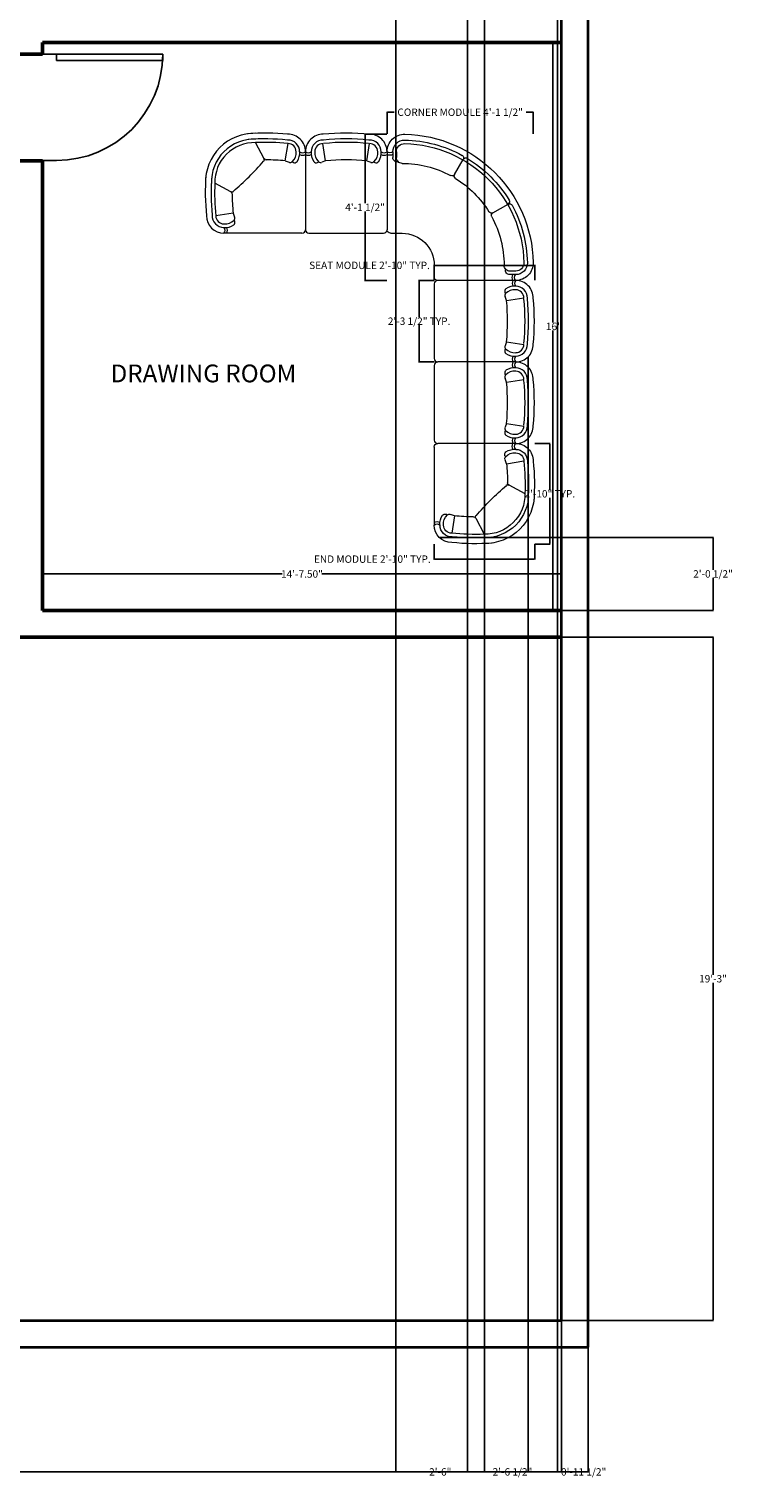
# Model space of a CAD drawing. Units: inches. Extents: x 594 to 1173, y 353 to 1285.
# Tile 3 of 6: x 934 to 1172, y 353 to 844. Entities that reach past the tile are written whole.
import ezdxf

# ---------------------------------------------------------------- set-up
doc = ezdxf.new("R2010")
doc.units = ezdxf.units.IN
doc.header["$MEASUREMENT"] = 0
for name, color, linetype, lineweight in [('A-ANNO-DIMS', 2, 'Continuous', 18), ('A-AREA-IDEN', 7, 'Continuous', 25), ('A-DOOR', 4, 'Continuous', 25), ('A-FURN', 8, 'Continuous', 18), ('A-WALL', 7, 'Continuous', 50), ('C-PROP', 7, 'Continuous', 35)]:
    doc.layers.add(name, color=color, linetype=linetype, lineweight=lineweight)
doc.styles.get("Standard").update_dxf_attribs({"font": 'arial.ttf'})
doc.dimstyles.get("Standard").update_dxf_attribs({"dimtxt": 2.5, "dimasz": 0.18, "dimexe": 0.18, "dimexo": 0.0625, "dimgap": 0.09, "dimtad": 0, "dimtih": 1, "dimtoh": 1, "dimzin": 0, "dimdsep": 46, "dimlunit": 3, "dimtxsty": 'Standard', "dimcen": 0.09, "dimadec": 0, "dimazin": 0, "dimtfac": 1, "dimtofl": 0, "dimtmove": 0, "dimatfit": 3, "dimfxl": 1, "dimtolj": 1, "dimtzin": 0, "dimarcsym": 0})

# ---------------------------------------------------------------- blocks, each defined once
blk = doc.blocks.new('*U2')
for p, q in [((0, 0), (0, -100)), ((750, 0), (750, -100))]:
    blk.add_line(p, q)
blk.add_lwpolyline([(0, 0), (0, 750), (43.75, 750), (43.75, 0)], close=True)
blk.add_arc((0, 0), 750, 0, 90)
blk = doc.blocks.new('A$C707258B2')
at = {"color": 0}
for p, q in [((0.404, 0.342), (1.074, 0.342)), ((0.404, 0.292), (0.454, 0.292)), ((0.404, 0.262), (0.454, 0.262)), ((1.104, 0.312), (1.104, 0.212)), ((1.479, -0.063), (1.379, -0.063)), ((1.509, -0.763), (1.509, -0.093)), ((0.6, -0.238), (0.47, -0.313)), ((0.929, -0.567), (0.854, -0.697)), ((1.429, -0.763), (1.429, -0.713)), ((1.459, -0.763), (1.459, -0.712))]:
    blk.add_line(p, q, dxfattribs=at)
for centre, radius, start, end in [((0.404, 0.192), 0.15, 90, 181.1754), ((0.404, 0.192), 0.1, 90, 181.1754), ((0.404, 0.192), 0.07, 90, 181.1754), ((0.378, 0.317), 0.0362, 316.3972, 43.6028), ((0.368, 0.317), 0.0662, 337.8298, 22.1702), ((0.455, 0.256), 0.0357, 345.4262, 90.5555), ((0.454, 0.212), 0.05, 360, 90), ((1.074, 0.312), 0.03, 360, 90), ((1.379, 0.212), 1.125, 181.1754, 268.8246), ((1.379, 0.212), 1.075, 181.1754, 208.6357), ((1.379, 0.212), 1.045, 181.1754, 268.8246), ((1.379, 0.212), 0.875, 180, 208.4082), ((1.379, 0.212), 0.275, 180, 270), ((1.479, -0.093), 0.03, 360, 90), ((0.587, -0.216), 0.025, 300, 28.4082), ((0.612, -0.259), 0.025, 31.5918, 120), ((1.379, 0.212), 0.875, 211.5918, 238.4082), ((0.457, -0.291), 0.025, 208.6357, 300), ((0.482, -0.334), 0.025, 120, 211.3643), ((1.379, 0.212), 1.075, 211.3643, 238.6357), ((0.907, -0.555), 0.025, 330, 58.4082), ((0.951, -0.58), 0.025, 61.5918, 150), ((1.379, 0.212), 0.875, 241.5918, 270), ((0.832, -0.685), 0.025, 238.6357, 330), ((0.876, -0.71), 0.025, 150, 241.3643), ((1.379, 0.212), 1.075, 241.3643, 268.8246), ((1.379, -0.713), 0.05, 360, 90), ((1.425, -0.709), 0.0336, 354.6301, 109.3883), ((1.484, -0.799), 0.0662, 67.8298, 112.1702), ((1.359, -0.763), 0.15, 268.8246, 360), ((1.359, -0.763), 0.1, 268.8246, 360), ((1.359, -0.763), 0.07, 268.8246, 360), ((1.484, -0.789), 0.0362, 46.3972, 133.6028)]:
    blk.add_arc(centre, radius, start, end, dxfattribs=at)
blk = doc.blocks.new('part 01')
at = {"color": 0}
for p, q in [((-670, 700), (0, 700)), ((30, 30), (30, 670)), ((-591, 527), (-740, 550)), ((-591, 527), (-579, 561)), ((-591, 173), (-740, 150)), ((-591, 173), (-579, 139)), ((-670, 0), (0, 0))]:
    blk.add_line(p, q, dxfattribs=at)
for centre, radius, start, end in [((-670, 550), 150, 90, 181.1754), ((-670, 550), 100, 90, 181.1754), ((-660, 518), 133, 56.0897, 95.6132), ((-696, 675), 36.2, 316.3972, 43.6028), ((-706, 675), 66.2, 337.8298, 22.1702), ((-600, 607), 25, 332.9608, 56.0897), ((0, 670), 30, 0, 90), ((1178, 350), 2008, 174.2835, 185.7165), ((1178, 350), 1958, 174.2835, 185.7165), ((1178, 350), 1928, 174.2835, 185.7165), ((-670, 550), 70, 90, 181.1754), ((-660, 518), 103, 42.0066, 95.6132), ((1178, 350), 1778, 174.2835, 185.7165), ((-625, 620), 53.2, 321.0017, 332.9608), ((-602, 570), 25, 340, 42.0066), ((-670, 150), 150, 178.8246, 270), ((-670, 150), 100, 178.8246, 270), ((-670, 150), 70, 178.8246, 270), ((-602, 130), 25, 317.9934, 20), ((-660, 182), 133, 264.3868, 303.9103), ((-660, 182), 103, 264.3868, 317.9934), ((-696, 25), 36.2, 316.3972, 43.6028), ((-706, 25), 66.2, 337.8298, 22.1702), ((-600, 93), 25, 303.9103, 27.0392), ((-625, 80), 53.2, 27.0392, 38.9983), ((0, 30), 30, 270, 0)]:
    blk.add_arc(centre, radius, start, end, dxfattribs=at)
blk = doc.blocks.new('part02')
at = {"color": 0}
for p, q in [((0, -670), (0, 0)), ((30, 30), (700, 30)), ((621, -143), (609, -109)), ((621, -143), (770, -120)), ((640, -326), (778, -399)), ((173, -591), (139, -579)), ((173, -591), (150, -740)), ((356, -610), (429, -748))]:
    blk.add_line(p, q, dxfattribs=at)
for centre, radius, start, end in [((30, 0), 30, 90, 180), ((726, 5), 56.2, 153.6122, 206.6666), ((726, 5), 36.2, 136.3972, 223.6028), ((700, -120), 150, 0, 90), ((630, -63), 25, 123.9103, 207.0392), ((655, -50), 53.2, 207.0392, 218.9983), ((632, -100), 25, 137.9934, 200), ((690, -152), 103, 84.3868, 137.9934), ((689, -151), 132, 85.4378, 123.9887), ((700, -121), 101, 357.5006, 89.858), ((700, -120), 70, 0, 90), ((-1228, -320), 2008, 357.7349, 5.7032), ((-1148, -320), 2008, 355.818, 5.7165), ((-1148, -320), 1778, 0.3836, 5.7165), ((-1148, -320), 1958, 355.8657, 5.7165), ((2220, -2190), 2454, 130.6961, 139.3039), ((632, -344), 20, 62, 130.6961), ((650, -308), 20, 180.3836, 242), ((439, -409), 419, 268.2181, 1.7819), ((439, -409), 369, 268.2181, 1.7819), ((439, -409), 339, 268.2181, 1.7819), ((182, -660), 133, 146.0897, 185.6132), ((93, -600), 25, 62.9608, 146.0897), ((182, -660), 103, 132.0066, 185.6132), ((80, -625), 53.2, 51.0017, 62.9608), ((130, -602), 25, 70, 132.0066), ((350, 1178), 1778, 264.2835, 269.6164), ((338, -620), 20, 28, 89.6164), ((374, -602), 20, 139.3039, 208), ((25, -696), 56.2, 63.3334, 116.3878), ((25, -696), 36.2, 46.3972, 133.6028), ((150, -670), 150, 180, 271.1754), ((150, -670), 100, 180, 271.1754), ((150, -670), 70, 180, 270), ((350, 1258), 2008, 264.2968, 272.2651), ((350, 1178), 2008, 264.2835, 274.182), ((350, 1178), 1958, 264.2835, 274.1343)]:
    blk.add_arc(centre, radius, start, end, dxfattribs=at)
blk = doc.blocks.new('*D19')
at = {"layer": 'A-ANNO-DIMS', "color": 0, "lineweight": -2, "transparency": 16777216}
for p, q in [((1114.27, 839.78), (1111.25, 839.78)), ((1111.43, 839.6), (1111.43, 745.15)), ((1111.43, 647.96), (1111.43, 742.42)), ((1114.27, 647.78), (1111.25, 647.78))]:
    blk.add_line(p, q, dxfattribs=at)
at = {"layer": 'A-ANNO-DIMS', "color": 0, "transparency": 16777216}
for points in [[(1111.4, 839.6), (1111.46, 839.6), (1111.43, 839.78)], [(1111.4, 647.96), (1111.46, 647.96), (1111.43, 647.78)]]:
    blk.add_solid(points, dxfattribs=at)
at = {"layer": 'Defpoints', "color": 0, "transparency": 16777216}
for p in [(1114.34, 839.78), (1111.43, 647.78), (1114.34, 647.78)]:
    blk.add_point(p, dxfattribs=at)
at = {"layer": 'A-ANNO-DIMS', "color": 0, "transparency": 16777216, "insert": (1111.43, 743.78), "char_height": 2.5, "attachment_point": 5}
blk.add_mtext("\\A1;16'", dxfattribs=at)
blk = doc.blocks.new('*D20')
at = {"layer": 'A-ANNO-DIMS', "color": 0, "lineweight": -2, "transparency": 16777216}
for p, q in [((938.84, 647.85), (938.84, 660.27)), ((939.02, 660.09), (1019.89, 660.09)), ((1114.16, 660.09), (1033.28, 660.09)), ((1114.34, 647.85), (1114.34, 660.27))]:
    blk.add_line(p, q, dxfattribs=at)
at = {"layer": 'A-ANNO-DIMS', "color": 0, "transparency": 16777216}
for points in [[(939.02, 660.12), (939.02, 660.06), (938.84, 660.09)], [(1114.16, 660.12), (1114.16, 660.06), (1114.34, 660.09)]]:
    blk.add_solid(points, dxfattribs=at)
at = {"layer": 'Defpoints', "color": 0, "transparency": 16777216}
for p in [(1114.34, 660.09), (938.84, 647.78), (1114.34, 647.78)]:
    blk.add_point(p, dxfattribs=at)
at = {"layer": 'A-ANNO-DIMS', "color": 0, "transparency": 16777216, "insert": (1026.59, 660.09), "char_height": 2.5, "attachment_point": 5}
blk.add_mtext('\\A1;14\'-7.50"', dxfattribs=at)
blk = doc.blocks.new('*D38')
at = {"layer": 'A-ANNO-DIMS', "color": 0, "lineweight": -2, "transparency": 16777216}
for p, q in [((1071.29, 764.42), (1071.11, 764.42)), ((1071.29, 759.38), (1071.29, 764.6)), ((1105.1, 764.42), (1071.47, 764.42)), ((1105.28, 759.38), (1105.28, 764.6))]:
    blk.add_line(p, q, dxfattribs=at)
at = {"layer": 'A-ANNO-DIMS', "color": 0, "transparency": 16777216}
for points in [[(1071.47, 764.45), (1071.47, 764.39), (1071.29, 764.42)], [(1105.1, 764.45), (1105.1, 764.39), (1105.28, 764.42)]]:
    blk.add_solid(points, dxfattribs=at)
at = {"layer": 'Defpoints', "color": 0, "transparency": 16777216}
for p in [(1071.29, 764.42), (1071.29, 759.32), (1105.28, 759.32)]:
    blk.add_point(p, dxfattribs=at)
at = {"layer": 'A-ANNO-DIMS', "color": 0, "transparency": 16777216, "insert": (1049.43, 764.42), "char_height": 2.5, "attachment_point": 5}
blk.add_mtext('\\A1;SEAT MODULE 2\'-10" TYP.', dxfattribs=at)
blk = doc.blocks.new('*D39')
at = {"layer": 'A-ANNO-DIMS', "color": 0, "lineweight": -2, "transparency": 16777216}
for p, q in [((1071.23, 759.32), (1066.01, 759.32)), ((1066.19, 759.14), (1066.19, 746.92)), ((1066.19, 731.94), (1066.19, 744.15)), ((1071.23, 731.76), (1066.01, 731.76))]:
    blk.add_line(p, q, dxfattribs=at)
at = {"layer": 'A-ANNO-DIMS', "color": 0, "transparency": 16777216}
for points in [[(1066.16, 759.14), (1066.22, 759.14), (1066.19, 759.32)], [(1066.16, 731.94), (1066.22, 731.94), (1066.19, 731.76)]]:
    blk.add_solid(points, dxfattribs=at)
at = {"layer": 'Defpoints', "color": 0, "transparency": 16777216}
for p in [(1071.29, 759.32), (1066.19, 731.76), (1071.29, 731.76)]:
    blk.add_point(p, dxfattribs=at)
at = {"layer": 'A-ANNO-DIMS', "color": 0, "transparency": 16777216, "insert": (1066.19, 745.54), "char_height": 2.5, "attachment_point": 5}
blk.add_mtext('\\A1;2\'-3 1/2" TYP.', dxfattribs=at)
blk = doc.blocks.new('*D40')
at = {"layer": 'A-ANNO-DIMS', "color": 0, "lineweight": -2, "transparency": 16777216}
for p, q in [((1071.29, 670.15), (1071.29, 664.94)), ((1105.27, 670.15), (1105.27, 664.94)), ((1071.29, 665.12), (1071.11, 665.12)), ((1105.09, 665.12), (1071.47, 665.12))]:
    blk.add_line(p, q, dxfattribs=at)
at = {"layer": 'A-ANNO-DIMS', "color": 0, "transparency": 16777216}
for points in [[(1071.47, 665.15), (1071.47, 665.09), (1071.29, 665.12)], [(1105.09, 665.15), (1105.09, 665.09), (1105.27, 665.12)]]:
    blk.add_solid(points, dxfattribs=at)
at = {"layer": 'Defpoints', "color": 0, "transparency": 16777216}
for p in [(1071.29, 670.21), (1105.27, 670.21), (1071.29, 665.12)]:
    blk.add_point(p, dxfattribs=at)
at = {"layer": 'A-ANNO-DIMS', "color": 0, "transparency": 16777216, "insert": (1050.37, 665.12), "char_height": 2.5, "attachment_point": 5}
blk.add_mtext('\\A1;END MODULE 2\'-10" TYP.', dxfattribs=at)
blk = doc.blocks.new('*D41')
at = {"layer": 'A-ANNO-DIMS', "color": 0, "lineweight": -2, "transparency": 16777216}
for p, q in [((1105.33, 704.19), (1110.54, 704.19)), ((1110.36, 704.01), (1110.36, 688.57)), ((1110.36, 670.39), (1110.36, 685.84)), ((1105.33, 670.21), (1110.54, 670.21))]:
    blk.add_line(p, q, dxfattribs=at)
at = {"layer": 'A-ANNO-DIMS', "color": 0, "transparency": 16777216}
for points in [[(1110.33, 704.01), (1110.39, 704.01), (1110.36, 704.19)], [(1110.33, 670.39), (1110.39, 670.39), (1110.36, 670.21)]]:
    blk.add_solid(points, dxfattribs=at)
at = {"layer": 'Defpoints', "color": 0, "transparency": 16777216}
for p in [(1105.27, 704.19), (1105.27, 670.21), (1110.36, 670.21)]:
    blk.add_point(p, dxfattribs=at)
at = {"layer": 'A-ANNO-DIMS', "color": 0, "transparency": 16777216, "insert": (1110.36, 687.2), "char_height": 2.5, "attachment_point": 5}
blk.add_mtext('\\A1;2\'-10" TYP.', dxfattribs=at)
blk = doc.blocks.new('*D42')
at = {"layer": 'A-ANNO-DIMS', "color": 0, "lineweight": -2, "transparency": 16777216}
for p, q in [((1055.34, 808.83), (1055.34, 816.36)), ((1055.52, 816.18), (1057.74, 816.18)), ((1104.6, 816.18), (1102.38, 816.18)), ((1104.78, 808.83), (1104.78, 816.36))]:
    blk.add_line(p, q, dxfattribs=at)
at = {"layer": 'A-ANNO-DIMS', "color": 0, "transparency": 16777216}
for points in [[(1055.52, 816.21), (1055.52, 816.15), (1055.34, 816.18)], [(1104.6, 816.21), (1104.6, 816.15), (1104.78, 816.18)]]:
    blk.add_solid(points, dxfattribs=at)
at = {"layer": 'Defpoints', "color": 0, "transparency": 16777216}
for p in [(1055.34, 816.18), (1055.34, 808.76), (1104.78, 808.76)]:
    blk.add_point(p, dxfattribs=at)
at = {"layer": 'A-ANNO-DIMS', "color": 0, "transparency": 16777216, "insert": (1080.06, 816.18), "char_height": 2.5, "attachment_point": 5}
blk.add_mtext('\\A1;CORNER MODULE 4\'-1 1/2"', dxfattribs=at)
blk = doc.blocks.new('*D43')
at = {"layer": 'A-ANNO-DIMS', "color": 0, "lineweight": -2, "transparency": 16777216}
for p, q in [((1055.28, 808.76), (1047.74, 808.76)), ((1047.92, 808.58), (1047.92, 785.42)), ((1047.92, 759.5), (1047.92, 782.66)), ((1055.28, 759.32), (1047.74, 759.32))]:
    blk.add_line(p, q, dxfattribs=at)
at = {"layer": 'A-ANNO-DIMS', "color": 0, "transparency": 16777216}
for points in [[(1047.89, 808.58), (1047.95, 808.58), (1047.92, 808.76)], [(1047.89, 759.5), (1047.95, 759.5), (1047.92, 759.32)]]:
    blk.add_solid(points, dxfattribs=at)
at = {"layer": 'Defpoints', "color": 0, "transparency": 16777216}
for p in [(1055.34, 808.76), (1047.92, 759.32), (1055.34, 759.32)]:
    blk.add_point(p, dxfattribs=at)
at = {"layer": 'A-ANNO-DIMS', "color": 0, "transparency": 16777216, "insert": (1047.92, 784.04), "char_height": 2.5, "attachment_point": 5}
blk.add_mtext('\\A1;4\'-1 1/2"', dxfattribs=at)
blk = doc.blocks.new('*D46')
at = {"layer": 'A-ANNO-DIMS', "color": 0, "lineweight": -2, "transparency": 16777216}
for p, q in [((643.34, 398.72), (643.34, 356.4)), ((1123.34, 398.72), (1123.34, 356.4)), ((643.52, 356.58), (878.9, 356.58)), ((1123.16, 356.58), (887.77, 356.58))]:
    blk.add_line(p, q, dxfattribs=at)
at = {"layer": 'A-ANNO-DIMS', "color": 0, "transparency": 16777216}
for points in [[(643.52, 356.61), (643.52, 356.55), (643.34, 356.58)], [(1123.16, 356.61), (1123.16, 356.55), (1123.34, 356.58)]]:
    blk.add_solid(points, dxfattribs=at)
at = {"layer": 'Defpoints', "color": 0, "transparency": 16777216}
for p in [(643.34, 398.78), (1123.34, 398.78), (1123.34, 356.58)]:
    blk.add_point(p, dxfattribs=at)
at = {"layer": 'A-ANNO-DIMS', "color": 0, "transparency": 16777216, "insert": (883.34, 356.58), "char_height": 2.5, "attachment_point": 5}
blk.add_mtext('\\A1;40\'-0"', dxfattribs=at)
blk = doc.blocks.new('*D62')
at = {"layer": 'A-ANNO-DIMS', "color": 0, "lineweight": -2, "transparency": 16777216}
for p, q in [((1082.5, 891.79), (1082.5, 356.4)), ((1113.01, 891.79), (1113.01, 356.4)), ((1082.68, 356.58), (1091.41, 356.58)), ((1112.83, 356.58), (1104.1, 356.58))]:
    blk.add_line(p, q, dxfattribs=at)
at = {"layer": 'A-ANNO-DIMS', "color": 0, "transparency": 16777216}
for points in [[(1082.68, 356.61), (1082.68, 356.55), (1082.5, 356.58)], [(1112.83, 356.61), (1112.83, 356.55), (1113.01, 356.58)]]:
    blk.add_solid(points, dxfattribs=at)
at = {"layer": 'Defpoints', "color": 0, "transparency": 16777216}
for p in [(1082.5, 891.85), (1113.01, 891.85), (1113.01, 356.58)]:
    blk.add_point(p, dxfattribs=at)
at = {"layer": 'A-ANNO-DIMS', "color": 0, "transparency": 16777216, "insert": (1097.75, 356.58), "char_height": 2.5, "attachment_point": 5}
blk.add_mtext('\\A1;2\'-6 1/2"', dxfattribs=at)
blk = doc.blocks.new('*D67')
at = {"layer": 'A-ANNO-DIMS', "color": 0, "lineweight": -2, "transparency": 16777216}
for p, q in [((1058.34, 1093.22), (1058.34, 356.4)), ((1088.34, 1093.22), (1088.34, 356.4)), ((1058.52, 356.58), (1069.9, 356.58)), ((1088.16, 356.58), (1076.77, 356.58))]:
    blk.add_line(p, q, dxfattribs=at)
at = {"layer": 'A-ANNO-DIMS', "color": 0, "transparency": 16777216}
for points in [[(1058.52, 356.61), (1058.52, 356.55), (1058.34, 356.58)], [(1088.16, 356.61), (1088.16, 356.55), (1088.34, 356.58)]]:
    blk.add_solid(points, dxfattribs=at)
at = {"layer": 'Defpoints', "color": 0, "transparency": 16777216}
for p in [(1058.34, 1093.28), (1088.34, 1093.28), (1058.34, 356.58)]:
    blk.add_point(p, dxfattribs=at)
at = {"layer": 'A-ANNO-DIMS', "color": 0, "transparency": 16777216, "insert": (1073.34, 356.58), "char_height": 2.5, "attachment_point": 5}
blk.add_mtext('\\A1;2\'-6"', dxfattribs=at)
blk = doc.blocks.new('*D80')
at = {"layer": 'A-ANNO-DIMS', "color": 0, "lineweight": -2, "transparency": 16777216}
for p, q in [((1103.07, 733.47), (1103.07, 356.4)), ((1114.34, 647.72), (1114.34, 356.4)), ((1103.25, 356.58), (1114.16, 356.58)), ((1114.34, 356.58), (1114.52, 356.58))]:
    blk.add_line(p, q, dxfattribs=at)
at = {"layer": 'A-ANNO-DIMS', "color": 0, "transparency": 16777216}
for points in [[(1103.25, 356.61), (1103.25, 356.55), (1103.07, 356.58)], [(1114.16, 356.61), (1114.16, 356.55), (1114.34, 356.58)]]:
    blk.add_solid(points, dxfattribs=at)
at = {"layer": 'Defpoints', "color": 0, "transparency": 16777216}
for p in [(1103.07, 733.53), (1114.34, 647.78), (1114.34, 356.58)]:
    blk.add_point(p, dxfattribs=at)
at = {"layer": 'A-ANNO-DIMS', "color": 0, "transparency": 16777216, "insert": (1121.81, 356.58), "char_height": 2.5, "attachment_point": 5}
blk.add_mtext('\\A1;0\'-11 1/2"', dxfattribs=at)
blk = doc.blocks.new('*D81')
at = {"layer": 'A-ANNO-DIMS', "color": 0, "lineweight": -2, "transparency": 16777216}
for p, q in [((1073.08, 672.46), (1165.72, 672.46)), ((1165.54, 672.28), (1165.54, 661.5)), ((1165.54, 647.96), (1165.54, 658.74)), ((1114.4, 647.78), (1165.72, 647.78))]:
    blk.add_line(p, q, dxfattribs=at)
at = {"layer": 'A-ANNO-DIMS', "color": 0, "transparency": 16777216}
for points in [[(1165.51, 672.28), (1165.57, 672.28), (1165.54, 672.46)], [(1165.51, 647.96), (1165.57, 647.96), (1165.54, 647.78)]]:
    blk.add_solid(points, dxfattribs=at)
at = {"layer": 'Defpoints', "color": 0, "transparency": 16777216}
for p in [(1073.02, 672.46), (1114.34, 647.78), (1165.54, 647.78)]:
    blk.add_point(p, dxfattribs=at)
at = {"layer": 'A-ANNO-DIMS', "color": 0, "transparency": 16777216, "insert": (1165.54, 660.12), "char_height": 2.5, "attachment_point": 5}
blk.add_mtext('\\A1;2\'-0 1/2"', dxfattribs=at)
blk = doc.blocks.new('*D83')
at = {"layer": 'A-ANNO-DIMS', "color": 0, "lineweight": -2, "transparency": 16777216}
for p, q in [((1114.4, 638.78), (1165.72, 638.78)), ((1165.54, 638.6), (1165.54, 524.65)), ((1165.54, 407.96), (1165.54, 521.92)), ((1114.4, 407.78), (1165.72, 407.78))]:
    blk.add_line(p, q, dxfattribs=at)
at = {"layer": 'A-ANNO-DIMS', "color": 0, "transparency": 16777216}
for points in [[(1165.51, 638.6), (1165.57, 638.6), (1165.54, 638.78)], [(1165.51, 407.96), (1165.57, 407.96), (1165.54, 407.78)]]:
    blk.add_solid(points, dxfattribs=at)
at = {"layer": 'Defpoints', "color": 0, "transparency": 16777216}
for p in [(1114.34, 638.78), (1165.54, 638.78), (1114.34, 407.78)]:
    blk.add_point(p, dxfattribs=at)
at = {"layer": 'A-ANNO-DIMS', "color": 0, "transparency": 16777216, "insert": (1165.54, 523.28), "char_height": 2.5, "attachment_point": 5}
blk.add_mtext('\\A1;19\'-3"', dxfattribs=at)

msp = doc.modelspace()

# ---------------------------------------------------------------- linework, layer by layer
at = {"layer": 'A-WALL'}
for p, q in [((938.837, 835.783), (929.837, 835.783)), ((938.837, 839.783), (1114.337, 839.783)), ((938.837, 835.783), (938.837, 839.783)), ((929.837, 799.783), (938.837, 799.783)), ((938.837, 647.783), (938.837, 799.862)), ((938.837, 647.783), (1114.337, 647.783)), ((820.337, 638.783), (1114.337, 638.783))]:
    msp.add_line(p, q, dxfattribs=at)
at = {"layer": 'C-PROP'}
for p, q in [((1123.337, 398.783), (1123.337, 1238.783)), ((1114.337, 407.783), (1114.337, 1062.283)), ((652.337, 407.783), (1114.337, 407.783)), ((643.337, 398.783), (1123.337, 398.783))]:
    msp.add_line(p, q, dxfattribs=at)

# ---------------------------------------------------------------- block references
at = {"layer": 'A-DOOR', "xscale": 0.0478936875771171, "yscale": 0.0478936875771171, "zscale": 0.0478936875771171, "rotation": 270}
msp.add_blockref('*U2', (943.626, 835.783), dxfattribs=at)
at = {"layer": 'A-FURN', "ltscale": 0.03}
for name, p, xscale, yscale, zscale, rotation in [('part02', (1027.776, 776.45), 0.0393782279651584, 0.0393782279651584, 0.0393782279651584, 180), ('part 01', (1027.776, 776.45), 0.0393782279651584, 0.0393782279651584, 0.0393782279651584, 270), ('A$C707258B2', (1068.809, 818.74), -39.37822796515838, 39.37822796515838, 39.37822796515838, 89.9999999999967), ('part 01', (1072.471, 759.321), 0.0393782279651584, 0.0393782279651584, 0.0393782279651584, 180), ('part 01', (1072.471, 731.756), 0.0393782279651584, 0.0393782279651584, 0.0393782279651584, 180), ('part02', (1072.471, 704.191), -0.0393782279651584, 0.0393782279651584, 0.0393782279651584, 89.9999999999967)]:
    msp.add_blockref(name, p, dxfattribs=dict(at, xscale=xscale, yscale=yscale, zscale=zscale, rotation=rotation))

# ---------------------------------------------------------------- texts
at = {"layer": 'A-AREA-IDEN'}
msp.add_text('DRAWING ROOM', height=6, dxfattribs=at).set_placement((961.9, 724.882))

# ---------------------------------------------------------------- dimensions: what is measured, and where the dimension line sits
at = {"layer": 'A-ANNO-DIMS'}
for base, p1, p2, override, picture, middle in [((1058.337, 356.583), (1088.337, 1093.283), (1058.337, 1093.283), {"dimdec": 1, "dimlfac": 1, "dimrnd": 0, "dimzin": 1, "dimdsep": 46, "dimlunit": 4, "dimfrac": 2}, '*D67', (1073.337, 356.583)), ((1113.008, 356.583), (1082.501, 891.849), (1113.008, 891.849), {"dimdec": 1, "dimlfac": 1, "dimrnd": 0, "dimzin": 1, "dimdsep": 46, "dimlunit": 4, "dimfrac": 2}, '*D62', (1097.755, 356.583)), ((1114.337, 356.583), (1103.065, 733.529), (1114.337, 647.783), {"dimdec": 1, "dimlfac": 1, "dimrnd": 0, "dimzin": 1, "dimdsep": 46, "dimlunit": 4, "dimfrac": 2}, '*D80', (1121.813, 356.583)), ((1114.337, 660.094), (938.837, 647.783), (1114.337, 647.783), {"dimclrd": 0, "dimclre": 0, "dimclrt": 0}, '*D20', (1026.587, 660.094)), ((1123.337, 356.583), (643.337, 398.783), (1123.337, 398.783), {"dimdec": 1, "dimlfac": 1, "dimrnd": 0, "dimzin": 1, "dimdsep": 46, "dimlunit": 4, "dimfrac": 2}, '*D46', (883.337, 356.583))]:
    dim = msp.add_linear_dim(base=base, p1=p1, p2=p2, dimstyle='Standard', override=override, dxfattribs=at)
    dim.commit()
    dim.dimension.update_dxf_attribs({"geometry": picture, "text_midpoint": middle})
for base, p1, p2, angle, override, picture, middle in [((1111.434, 647.783), (1114.337, 839.783), (1114.337, 647.783), 90, {"dimclrd": 0, "dimclre": 0, "dimclrt": 0}, '*D19', (1111.434, 743.783)), ((1047.925, 759.321), (1055.341, 808.764), (1055.341, 759.321), 270, {"dimdec": 1, "dimlfac": 1, "dimrnd": 0, "dimzin": 1, "dimdsep": 46, "dimlunit": 4, "dimfrac": 2}, '*D43', (1047.925, 784.042)), ((1165.537, 647.783), (1073.019, 672.458), (1114.337, 647.783), 90, {"dimdec": 1, "dimlfac": 1, "dimrnd": 0, "dimzin": 1, "dimdsep": 46, "dimlunit": 4, "dimfrac": 2}, '*D81', (1165.537, 660.12)), ((1165.537, 638.783), (1114.337, 407.783), (1114.337, 638.783), 90, {"dimdec": 1, "dimlfac": 1, "dimrnd": 0, "dimzin": 1, "dimdsep": 46, "dimlunit": 4, "dimfrac": 2}, '*D83', (1165.537, 523.283))]:
    dim = msp.add_linear_dim(base=base, p1=p1, p2=p2, angle=angle, dimstyle='Standard', override=override, dxfattribs=at)
    dim.commit()
    dim.dimension.update_dxf_attribs({"geometry": picture, "text_midpoint": middle})
for base, p1, p2, angle, text, picture, middle in [((1055.341, 816.18), (1104.784, 808.764), (1055.341, 808.764), 180, 'CORNER MODULE <>', '*D42', (1080.062, 816.18)), ((1071.289, 764.419), (1105.277, 759.321), (1071.289, 759.321), 180, 'SEAT MODULE <> TYP.', '*D38', (1049.432, 764.419)), ((1066.191, 731.756), (1071.289, 759.321), (1071.289, 731.756), 270, '<> TYP.', '*D39', (1066.191, 745.538)), ((1110.364, 670.213), (1105.268, 704.191), (1105.268, 670.213), 270, '<> TYP.', '*D41', (1110.364, 687.202)), ((1071.289, 665.116), (1105.268, 670.213), (1071.289, 670.213), 180, 'END MODULE <> TYP.', '*D40', (1050.366, 665.116))]:
    dim = msp.add_linear_dim(base=base, p1=p1, p2=p2, angle=angle, text=text, dimstyle='Standard', override={"dimdec": 1, "dimlfac": 1, "dimrnd": 0, "dimzin": 1, "dimdsep": 46, "dimlunit": 4, "dimfrac": 2}, dxfattribs=at)
    dim.commit()
    dim.dimension.update_dxf_attribs({"geometry": picture, "text_midpoint": middle})

doc.saveas('drawing.dxf')
